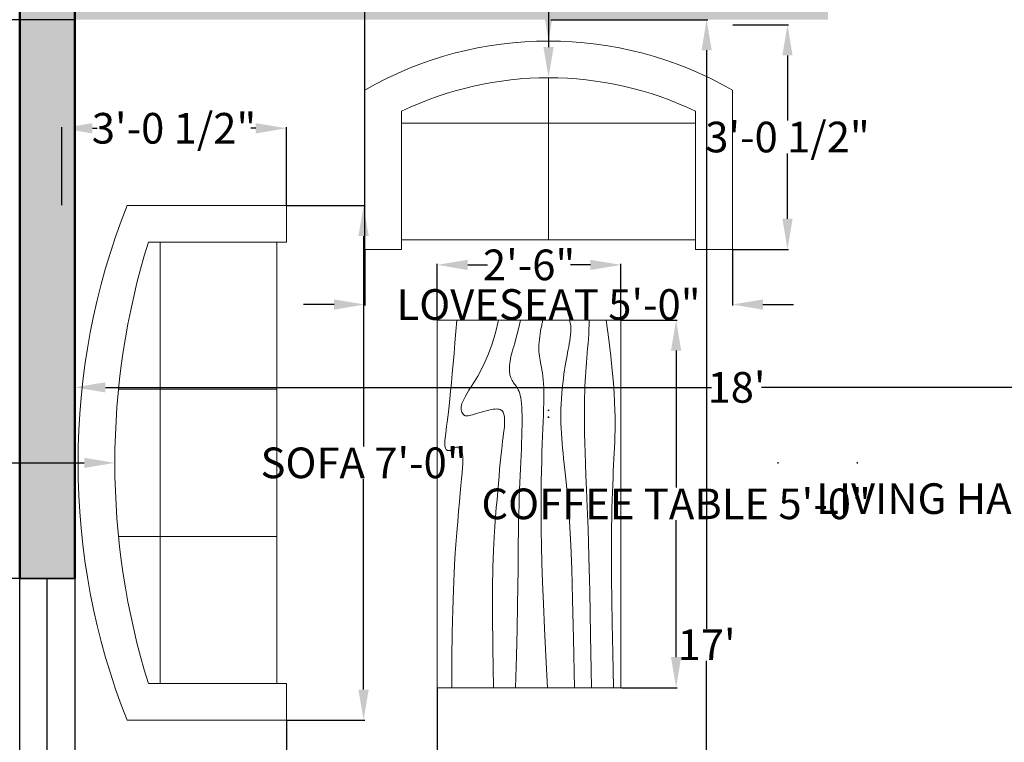
# Model space of a CAD drawing. Units: inches. Extents: x 3136 to 3620, y 13606 to 14152.
# Tile 3 of 6: x 3225 to 3386, y 13734 to 13852. Entities that reach past the tile are written whole.
import ezdxf

# ---------------------------------------------------------------- set-up
doc = ezdxf.new("R2010")
doc.units = ezdxf.units.IN
for name, color, linetype, lineweight in [('A-ANNO-DIMS', 2, 'Continuous', 18), ('A-AREA-IDEN', 7, 'Continuous', 25), ('A-FURN', 8, 'Continuous', 18), ('A-GLAZ', 4, 'Continuous', 25), ('A-WALL', 7, 'Continuous', 50), ('A-WALL-PATT', 174, 'Continuous', 13)]:
    doc.layers.add(name, color=color, linetype=linetype, lineweight=lineweight)
doc.styles.get("Standard").update_dxf_attribs({"font": 'arial.ttf', "height": 5})
doc.dimstyles.get("Standard").update_dxf_attribs({"dimtxt": 5, "dimasz": 5, "dimexe": 0.18, "dimexo": 0.0625, "dimgap": 0.09, "dimtad": 0, "dimtih": 1, "dimtoh": 1, "dimdec": 0, "dimzin": 0, "dimdsep": 46, "dimlunit": 3, "dimtxsty": 'Standard', "dimcen": 0.09, "dimadec": 0, "dimazin": 0, "dimtfac": 1, "dimtdec": 0, "dimtofl": 0, "dimtmove": 0, "dimatfit": 3, "dimfxl": 1, "dimtolj": 1, "dimtzin": 0, "dimarcsym": 0})

# ---------------------------------------------------------------- blocks, each defined once
blk = doc.blocks.new('*D15')
at = {"layer": 'A-ANNO-DIMS', "color": 0, "lineweight": -2, "transparency": 16777216}
for p, q in [((3233.87, 13788.87), (3233.87, 13792.02)), ((3238.87, 13791.84), (3337.77, 13791.84)), ((3444.87, 13791.84), (3345.97, 13791.84)), ((3449.87, 13788.87), (3449.87, 13792.02))]:
    blk.add_line(p, q, dxfattribs=at)
at = {"layer": 'A-ANNO-DIMS', "color": 0, "transparency": 16777216}
for points in [[(3238.87, 13792.67), (3238.87, 13791.01), (3233.87, 13791.84)], [(3444.87, 13792.67), (3444.87, 13791.01), (3449.87, 13791.84)]]:
    blk.add_solid(points, dxfattribs=at)
at = {"layer": 'Defpoints', "color": 0, "transparency": 16777216}
for p in [(3449.87, 13791.84), (3233.87, 13788.8), (3449.87, 13788.8)]:
    blk.add_point(p, dxfattribs=at)
at = {"layer": 'A-ANNO-DIMS', "color": 0, "transparency": 16777216, "insert": (3341.87, 13791.84), "char_height": 5, "attachment_point": 5}
blk.add_mtext("\\A1;18'", dxfattribs=at)
blk = doc.blocks.new('*D16')
at = {"layer": 'A-ANNO-DIMS', "color": 0, "lineweight": -2, "transparency": 16777216}
for p, q in [((3311.54, 13851.84), (3337.17, 13851.84)), ((3336.99, 13846.84), (3336.99, 13752.44)), ((3336.99, 13652.84), (3336.99, 13747.24)), ((3311.54, 13647.84), (3337.17, 13647.84))]:
    blk.add_line(p, q, dxfattribs=at)
at = {"layer": 'A-ANNO-DIMS', "color": 0, "transparency": 16777216}
for points in [[(3336.16, 13846.84), (3337.82, 13846.84), (3336.99, 13851.84)], [(3336.16, 13652.84), (3337.82, 13652.84), (3336.99, 13647.84)]]:
    blk.add_solid(points, dxfattribs=at)
at = {"layer": 'Defpoints', "color": 0, "transparency": 16777216}
for p in [(3311.47, 13851.84), (3336.99, 13851.84), (3311.47, 13647.84)]:
    blk.add_point(p, dxfattribs=at)
at = {"layer": 'A-ANNO-DIMS', "color": 0, "transparency": 16777216, "insert": (3336.99, 13749.84), "char_height": 5, "attachment_point": 5}
blk.add_mtext("\\A1;17'", dxfattribs=at)
blk = doc.blocks.new('Table - Rectangular Woodgrain 60 x 30 in.')
for p, q in [((0, 0), (0, -30)), ((60, 0), (0, 0)), ((60, -30), (60, 0)), ((0, -30), (60, -30))]:
    blk.add_line(p, q)
for points in [[(0, -2.4), (4.8155, -2.418), (9.0302, -2.4688), (12.709, -2.5477), (15.9167, -2.65), (18.7181, -2.7711), (21.1781, -2.9063), (23.3616, -3.0508), (25.3333, -3.2), (27.1477, -3.3495), (28.8172, -3.4958), (30.3437, -3.636), (31.7291, -3.7667), (32.9756, -3.8849), (34.0849, -3.9875), (35.059, -4.0714), (35.9, -4.1334), (36.6114, -4.1711), (37.2041, -4.1854), (37.6906, -4.1779), (38.0833, -4.15), (38.3948, -4.1034), (38.6375, -4.0396), (38.8239, -3.9602), (38.9666, -3.8667), (39.0764, -3.7608), (39.1573, -3.6448), (39.2116, -3.521), (39.2416, -3.3917), (39.2498, -3.2593), (39.2385, -3.1261), (39.21, -2.9944), (39.1666, -2.8667), (39.111, -2.7447), (39.0468, -2.6281), (38.978, -2.5163), (38.9083, -2.4083), (38.8418, -2.3035), (38.7823, -2.201), (38.7337, -2.1001), (38.7, -2), (38.6844, -1.9003), (38.6875, -1.8021), (38.7094, -1.707), (38.75, -1.6167), (38.8094, -1.5326), (38.8875, -1.4563), (38.9844, -1.3893), (39.1, -1.3333), (39.2351, -1.2896), (39.3937, -1.2583), (39.5804, -1.2396), (39.8, -1.2333), (40.057, -1.2396), (40.3562, -1.2583), (40.7023, -1.2896), (41.1, -1.3333), (41.5547, -1.3895), (42.0755, -1.4573), (42.6721, -1.5361), (43.3542, -1.625), (44.1316, -1.7233), (45.014, -1.8302), (46.0114, -1.9449), (47.1333, -2.0667), (48.3862, -2.1947), (49.7625, -2.3281), (51.2513, -2.4663), (52.8416, -2.6083), (54.5226, -2.7535), (56.2833, -2.9011), (58.1127, -3.0501), (60, -3.2)], [(0, -9.2), (6.5759, -9.0858), (11.9385, -9.0365), (16.2527, -9.0418), (19.6833, -9.0917), (22.3952, -9.1759), (24.5531, -9.2844), (26.322, -9.4069), (27.8666, -9.5333), (29.3241, -9.6553), (30.7203, -9.7719), (32.0532, -9.8837), (33.3208, -9.9917), (34.5213, -10.0965), (35.6526, -10.199), (36.7128, -10.2999), (37.7, -10.4), (38.6129, -10.4996), (39.4531, -10.5969), (40.223, -10.6895), (40.925, -10.775), (41.5613, -10.8512), (42.1344, -10.9156), (42.6465, -10.966), (43.1, -11), (43.4976, -11.0158), (43.8437, -11.0136), (44.143, -10.9942), (44.4, -10.9583), (44.6195, -10.9069), (44.8062, -10.8406), (44.9648, -10.7603), (45.1, -10.6667), (45.2155, -10.5598), (45.3114, -10.4365), (45.3871, -10.2929), (45.4416, -10.125), (45.4743, -9.929), (45.4844, -9.7011), (45.4709, -9.4371), (45.4333, -9.1333), (45.3716, -8.7883), (45.2896, -8.4104), (45.1919, -8.0107), (45.0833, -7.6), (44.9685, -7.1893), (44.8521, -6.7896), (44.7388, -6.4117), (44.6333, -6.0667), (44.54, -5.7628), (44.4614, -5.4979), (44.4001, -5.2675), (44.3583, -5.0667), (44.3384, -4.8909), (44.3427, -4.7354), (44.3736, -4.5956), (44.4333, -4.4667), (44.5236, -4.3453), (44.6427, -4.2333), (44.7884, -4.1339), (44.9583, -4.05), (45.1501, -3.9849), (45.3614, -3.9417), (45.59, -3.9234), (45.8333, -3.9333), (46.0915, -3.9749), (46.3734, -4.0531), (46.6906, -4.1736), (47.0542, -4.3417), (47.4756, -4.5629), (47.9661, -4.8427), (48.5372, -5.1866), (49.2, -5.6), (49.9676, -6.0844), (50.8594, -6.625), (51.8965, -7.2031), (53.1, -7.8), (54.491, -8.3969), (56.0906, -8.975), (57.9199, -9.5156), (60, -10)], [(0, -12.8), (5.1847, -12.9322), (9.6213, -13.0323), (13.3963, -13.1059), (16.5958, -13.1583), (19.3063, -13.1952), (21.614, -13.2219), (23.6054, -13.2439), (25.3666, -13.2667), (26.9728, -13.2947), (28.4531, -13.3281), (29.8256, -13.3663), (31.1083, -13.4083), (32.3191, -13.4535), (33.476, -13.501), (34.597, -13.5501), (35.7, -13.6), (36.7984, -13.6497), (37.8875, -13.6979), (38.9578, -13.743), (40, -13.7833), (41.0047, -13.8174), (41.9625, -13.8438), (42.864, -13.8607), (43.7, -13.8667), (44.4631, -13.8604), (45.1552, -13.8417), (45.7801, -13.8104), (46.3416, -13.7667), (46.8439, -13.7104), (47.2906, -13.6417), (47.6858, -13.5604), (48.0333, -13.4667), (48.3375, -13.3608), (48.6042, -13.2448), (48.8396, -13.121), (49.05, -12.9917), (49.2417, -12.8593), (49.4208, -12.7261), (49.5937, -12.5944), (49.7667, -12.4667), (49.9452, -12.3451), (50.1323, -12.2313), (50.3303, -12.1268), (50.5416, -12.0333), (50.7686, -11.9524), (51.0135, -11.8854), (51.2788, -11.8341), (51.5666, -11.8), (51.8785, -11.7843), (52.2116, -11.7865), (52.562, -11.8059), (52.926, -11.8417), (53.2998, -11.8931), (53.6795, -11.9594), (54.0614, -12.0397), (54.4416, -12.1333), (54.8223, -12.2401), (55.2293, -12.3625), (55.6942, -12.5037), (56.2489, -12.6667), (56.9251, -12.8547), (57.7545, -13.0708), (58.7689, -13.3182), (60, -13.6)], [(0, -18), (5.124, -17.7273), (9.6609, -17.5057), (13.6705, -17.3303), (17.2125, -17.1958), (20.3467, -17.0973), (23.1328, -17.0297), (25.6307, -16.9878), (27.9, -16.9667), (29.9928, -16.9617), (31.9302, -16.9703), (33.7254, -16.9907), (35.3917, -17.0208), (36.9423, -17.0588), (38.3906, -17.1026), (39.7499, -17.1503), (41.0333, -17.2), (42.2519, -17.2496), (43.4073, -17.2969), (44.4986, -17.3395), (45.525, -17.375), (46.4858, -17.4012), (47.3802, -17.4156), (48.2074, -17.416), (48.9667, -17.4), (49.6583, -17.3662), (50.2872, -17.3167), (50.8595, -17.2547), (51.3812, -17.1833), (51.8584, -17.1057), (52.2971, -17.025), (52.7034, -16.9443), (53.0833, -16.8667), (53.443, -16.7951), (53.789, -16.7313), (54.128, -16.6768), (54.4666, -16.6334), (54.8115, -16.6024), (55.1693, -16.5854), (55.5465, -16.5841), (55.95, -16.6), (56.3828, -16.6337), (56.8346, -16.6823), (57.2915, -16.7418), (57.7396, -16.8084), (58.165, -16.878), (58.5539, -16.9469), (58.8924, -17.0111), (59.1666, -17.0667), (59.3679, -17.1107), (59.5078, -17.1438), (59.6032, -17.1675), (59.6708, -17.1833), (59.7275, -17.193), (59.7901, -17.1979), (59.8753, -17.1998), (60, -17.2)], [(0, -22.4), (8.0098, -22.2501), (14.4094, -22.1011), (19.4168, -21.9535), (23.25, -21.8083), (26.1269, -21.6663), (28.2656, -21.5281), (29.884, -21.3947), (31.2, -21.2667), (32.3967, -21.1448), (33.5172, -21.0292), (34.5697, -20.9198), (35.5625, -20.8167), (36.5037, -20.7198), (37.4015, -20.6292), (38.2642, -20.5448), (39.1, -20.4667), (39.9164, -20.3951), (40.7187, -20.3313), (41.5117, -20.2768), (42.3, -20.2333), (43.0883, -20.2024), (43.8812, -20.1854), (44.6836, -20.1841), (45.5, -20.2), (46.3328, -20.234), (47.1747, -20.2844), (48.0163, -20.3488), (48.8479, -20.425), (49.66, -20.5106), (50.4429, -20.6031), (51.1872, -20.7004), (51.8833, -20.8), (52.5246, -20.8999), (53.1166, -20.9995), (53.6681, -21.0983), (54.1875, -21.1958), (54.6834, -21.2919), (55.1646, -21.3859), (55.6394, -21.4777), (56.1167, -21.5667), (56.6028, -21.6515), (57.0961, -21.7266), (57.5929, -21.7852), (58.0896, -21.8208), (58.5823, -21.8268), (59.0674, -21.7964), (59.5412, -21.723), (60, -21.6)], [(0, -25.2), (8.6355, -25.0504), (15.7026, -24.9031), (21.4049, -24.7606), (25.9458, -24.625), (29.529, -24.4988), (32.3578, -24.3844), (34.6359, -24.284), (36.5667, -24.2), (38.3213, -24.1341), (39.9417, -24.0854), (41.437, -24.0523), (42.8167, -24.0333), (44.0901, -24.0268), (45.2667, -24.0313), (46.3557, -24.0451), (47.3667, -24.0667), (48.309, -24.0947), (49.1928, -24.1287), (50.0284, -24.168), (50.826, -24.2125), (51.5959, -24.2617), (52.3483, -24.3151), (53.0935, -24.3725), (53.8417, -24.4334), (54.6009, -24.497), (55.3699, -24.561), (56.1454, -24.6226), (56.9239, -24.6792), (57.7021, -24.7279), (58.4764, -24.7662), (59.2435, -24.7911), (60, -24.8)], [(0, -28.8), (5.6867, -28.6681), (10.45, -28.5698), (14.407, -28.5012), (17.675, -28.4584), (20.3711, -28.4374), (22.6125, -28.4344), (24.5164, -28.4455), (26.2, -28.4667), (27.762, -28.4947), (29.2276, -28.5281), (30.6033, -28.5663), (31.8958, -28.6084), (33.1118, -28.6535), (34.2578, -28.7011), (35.3405, -28.7501), (36.3666, -28.8), (37.3443, -28.8497), (38.288, -28.8974), (39.2137, -28.9412), (40.1375, -28.9792), (41.0753, -29.0093), (42.0432, -29.0297), (43.0572, -29.0384), (44.1333, -29.0333), (45.2936, -29.0114), (46.5843, -28.9641), (48.0579, -28.8816), (49.7666, -28.7542), (51.7629, -28.5721), (54.0989, -28.3255), (56.8272, -28.0048), (60, -27.6)]]:
    blk.add_lwpolyline(points)
blk = doc.blocks.new('Sofa - Roundback 7 ft.')
for p, q in [((-12.00002, -32.4421), (-12.00003, -6.5971)), ((11.99997, -32.4421), (11.99998, -6.5971)), ((-36.000027, -34), (-36.000027, -11.4696)), ((35.99998, -34), (35.99998, -11.4696)), ((-35.999844, -13.3819), (35.9998, -13.3819)), ((-36.000027, -32.4421), (35.99998, -32.4421))]:
    blk.add_line(p, q)
for points in [[(-36.000027, -34), (-42.000027, -34), (-42.000027, -8)], [(41.99998, -8), (41.99998, -34), (35.99998, -34)]]:
    blk.add_lwpolyline(points)
for centre, radius, start, end in [((0, -114.25), 114.25, 68.43141, 111.5686), ((-0.00001, -127.1968), 121.1968, 72.72033, 107.2797)]:
    blk.add_arc(centre, radius, start, end)
blk = doc.blocks.new('Sofa - Roundback Loveseat 5 ft.')
for p, q in [((0, -32.44198), (0, -5.99998)), ((-24, -33.99998), (-24, -11.46958)), ((24.00004, -33.99998), (24.00004, -11.46958)), ((-23.9998, -13.38178), (23.99986, -13.38178)), ((-24, -32.44198), (24.00004, -32.44198))]:
    blk.add_line(p, q)
for points in [[(-24, -33.99998), (-30, -33.99998), (-30, -7.99998)], [(30.00004, -7.99998), (30.00004, -33.99998), (24.00004, -33.99998)]]:
    blk.add_lwpolyline(points)
for centre, radius, start, end in [((0, -60.24998), 60.24998, 60.13715, 119.8628), ((0, -61.38438), 55.38444, 64.32083, 115.6792)]:
    blk.add_arc(centre, radius, start, end)
blk = doc.blocks.new('*D28')
at = {"layer": 'A-ANNO-DIMS', "color": 0, "lineweight": -2, "transparency": 16777216}
for p, q in [((3224.81, 14118.84), (3200.37, 14118.84)), ((3200.55, 14113.84), (3200.55, 13881.48)), ((3200.55, 13643.84), (3200.55, 13876.2)), ((3224.81, 13638.84), (3200.37, 13638.84))]:
    blk.add_line(p, q, dxfattribs=at)
at = {"layer": 'A-ANNO-DIMS', "color": 0, "transparency": 16777216}
for points in [[(3199.71, 14113.84), (3201.38, 14113.84), (3200.55, 14118.84)], [(3199.71, 13643.84), (3201.38, 13643.84), (3200.55, 13638.84)]]:
    blk.add_solid(points, dxfattribs=at)
at = {"layer": 'Defpoints', "color": 0, "transparency": 16777216}
for p in [(3200.55, 14118.84), (3224.87, 14118.84), (3224.87, 13638.84)]:
    blk.add_point(p, dxfattribs=at)
at = {"layer": 'A-ANNO-DIMS', "color": 0, "transparency": 16777216, "insert": (3200.55, 13878.84), "char_height": 5, "attachment_point": 5}
blk.add_mtext("\\A1;40'", dxfattribs=at)
blk = doc.blocks.new('*D34')
at = {"layer": 'A-ANNO-DIMS', "color": 0, "lineweight": -2, "transparency": 16777216}
for p, q in [((3323.07, 13802.83), (3332.19, 13802.83)), ((3332.01, 13797.83), (3332.01, 13775.5)), ((3332.01, 13747.83), (3332.01, 13770.15)), ((3323.07, 13742.83), (3332.19, 13742.83))]:
    blk.add_line(p, q, dxfattribs=at)
at = {"layer": 'A-ANNO-DIMS', "color": 0, "transparency": 16777216}
for points in [[(3331.17, 13797.83), (3332.84, 13797.83), (3332.01, 13802.83)], [(3331.17, 13747.83), (3332.84, 13747.83), (3332.01, 13742.83)]]:
    blk.add_solid(points, dxfattribs=at)
at = {"layer": 'Defpoints', "color": 0, "transparency": 16777216}
for p in [(3323.01, 13802.83), (3332.01, 13802.83), (3323.01, 13742.83)]:
    blk.add_point(p, dxfattribs=at)
at = {"layer": 'A-ANNO-DIMS', "color": 0, "transparency": 16777216, "insert": (3332.01, 13772.83), "char_height": 5, "attachment_point": 5}
blk.add_mtext('\\A1;COFFEE TABLE 5\'-0"', dxfattribs=at)
blk = doc.blocks.new('*D35')
at = {"layer": 'A-ANNO-DIMS', "color": 0, "lineweight": -2, "transparency": 16777216}
for p, q in [((3293.01, 13802.89), (3293.01, 13812.01)), ((3298.01, 13811.83), (3301.23, 13811.83)), ((3318.01, 13811.83), (3314.79, 13811.83)), ((3323.01, 13802.89), (3323.01, 13812.01))]:
    blk.add_line(p, q, dxfattribs=at)
at = {"layer": 'A-ANNO-DIMS', "color": 0, "transparency": 16777216}
for points in [[(3298.01, 13812.66), (3298.01, 13810.99), (3293.01, 13811.83)], [(3318.01, 13812.66), (3318.01, 13810.99), (3323.01, 13811.83)]]:
    blk.add_solid(points, dxfattribs=at)
at = {"layer": 'Defpoints', "color": 0, "transparency": 16777216}
for p in [(3293.01, 13811.83), (3293.01, 13802.83), (3323.01, 13802.83)]:
    blk.add_point(p, dxfattribs=at)
at = {"layer": 'A-ANNO-DIMS', "color": 0, "transparency": 16777216, "insert": (3308.01, 13811.83), "char_height": 5, "attachment_point": 5}
blk.add_mtext('\\A1;2\'-6"', dxfattribs=at)
blk = doc.blocks.new('*D36')
at = {"layer": 'A-ANNO-DIMS', "color": 0, "lineweight": -2, "transparency": 16777216}
for p, q in [((3268.46, 13821.52), (3281.18, 13821.52)), ((3281, 13816.52), (3281, 13782.19)), ((3281, 13742.52), (3281, 13776.84)), ((3268.46, 13737.52), (3281.18, 13737.52))]:
    blk.add_line(p, q, dxfattribs=at)
at = {"layer": 'A-ANNO-DIMS', "color": 0, "transparency": 16777216}
for points in [[(3280.16, 13816.52), (3281.83, 13816.52), (3281, 13821.52)], [(3280.16, 13742.52), (3281.83, 13742.52), (3281, 13737.52)]]:
    blk.add_solid(points, dxfattribs=at)
at = {"layer": 'Defpoints', "color": 0, "transparency": 16777216}
for p in [(3268.4, 13821.52), (3281, 13821.52), (3268.4, 13737.52)]:
    blk.add_point(p, dxfattribs=at)
at = {"layer": 'A-ANNO-DIMS', "color": 0, "transparency": 16777216, "insert": (3281, 13779.52), "char_height": 5, "attachment_point": 5}
blk.add_mtext('\\A1;SOFA 7\'-0"', dxfattribs=at)
blk = doc.blocks.new('*D37')
at = {"layer": 'A-ANNO-DIMS', "color": 0, "lineweight": -2, "transparency": 16777216}
for p, q in [((3231.73, 13821.58), (3231.73, 13834.3)), ((3236.73, 13834.12), (3237.51, 13834.12)), ((3263.4, 13834.12), (3262.62, 13834.12)), ((3268.4, 13821.58), (3268.4, 13834.3))]:
    blk.add_line(p, q, dxfattribs=at)
at = {"layer": 'A-ANNO-DIMS', "color": 0, "transparency": 16777216}
for points in [[(3236.73, 13834.95), (3236.73, 13833.28), (3231.73, 13834.12)], [(3263.4, 13834.95), (3263.4, 13833.28), (3268.4, 13834.12)]]:
    blk.add_solid(points, dxfattribs=at)
at = {"layer": 'Defpoints', "color": 0, "transparency": 16777216}
for p in [(3231.73, 13834.12), (3231.73, 13821.52), (3268.4, 13821.52)]:
    blk.add_point(p, dxfattribs=at)
at = {"layer": 'A-ANNO-DIMS', "color": 0, "transparency": 16777216, "insert": (3250.06, 13834.12), "char_height": 5, "attachment_point": 5}
blk.add_mtext('\\A1;3\'-0 1/2"', dxfattribs=at)
blk = doc.blocks.new('*D38')
at = {"layer": 'A-ANNO-DIMS', "color": 0, "lineweight": -2, "transparency": 16777216}
for p, q in [((3281.19, 13814.29), (3281.19, 13805.18)), ((3341.19, 13814.29), (3341.19, 13805.18)), ((3276.19, 13805.36), (3271.19, 13805.36)), ((3346.19, 13805.36), (3351.19, 13805.36))]:
    blk.add_line(p, q, dxfattribs=at)
at = {"layer": 'A-ANNO-DIMS', "color": 0, "transparency": 16777216}
for points in [[(3276.19, 13806.19), (3276.19, 13804.52), (3281.19, 13805.36)], [(3346.19, 13806.19), (3346.19, 13804.52), (3341.19, 13805.36)]]:
    blk.add_solid(points, dxfattribs=at)
at = {"layer": 'Defpoints', "color": 0, "transparency": 16777216}
for p in [(3281.19, 13814.36), (3341.19, 13814.36), (3341.19, 13805.36)]:
    blk.add_point(p, dxfattribs=at)
at = {"layer": 'A-ANNO-DIMS', "color": 0, "transparency": 16777216, "insert": (3311.19, 13805.36), "char_height": 5, "attachment_point": 5}
blk.add_mtext('\\A1;LOVESEAT 5\'-0"', dxfattribs=at)
blk = doc.blocks.new('*D39')
at = {"layer": 'A-ANNO-DIMS', "color": 0, "lineweight": -2, "transparency": 16777216}
for p, q in [((3341.25, 13851.02), (3350.37, 13851.02)), ((3350.19, 13846.02), (3350.19, 13835.37)), ((3350.19, 13819.36), (3350.19, 13830.01)), ((3341.25, 13814.36), (3350.37, 13814.36))]:
    blk.add_line(p, q, dxfattribs=at)
at = {"layer": 'A-ANNO-DIMS', "color": 0, "transparency": 16777216}
for points in [[(3349.36, 13846.02), (3351.02, 13846.02), (3350.19, 13851.02)], [(3349.36, 13819.36), (3351.02, 13819.36), (3350.19, 13814.36)]]:
    blk.add_solid(points, dxfattribs=at)
at = {"layer": 'Defpoints', "color": 0, "transparency": 16777216}
for p in [(3341.19, 13851.02), (3350.19, 13851.02), (3341.19, 13814.36)]:
    blk.add_point(p, dxfattribs=at)
at = {"layer": 'A-ANNO-DIMS', "color": 0, "transparency": 16777216, "insert": (3350.19, 13832.69), "char_height": 5, "attachment_point": 5}
blk.add_mtext('\\A1;3\'-0 1/2"', dxfattribs=at)
blk = doc.blocks.new('*D63')
at = {"layer": 'A-ANNO-DIMS', "color": 0, "lineweight": -2, "transparency": 16777216}
for p, q in [((3233.81, 13851.84), (3207.89, 13851.84)), ((3208.07, 13846.84), (3208.07, 13808.82)), ((3208.07, 13765.63), (3208.07, 13803.64)), ((3233.81, 13760.63), (3207.89, 13760.63))]:
    blk.add_line(p, q, dxfattribs=at)
at = {"layer": 'A-ANNO-DIMS', "color": 0, "transparency": 16777216}
for points in [[(3207.24, 13846.84), (3208.9, 13846.84), (3208.07, 13851.84)], [(3207.24, 13765.63), (3208.9, 13765.63), (3208.07, 13760.63)]]:
    blk.add_solid(points, dxfattribs=at)
at = {"layer": 'Defpoints', "color": 0, "transparency": 16777216}
for p in [(3208.07, 13851.84), (3233.87, 13851.84), (3233.87, 13760.63)]:
    blk.add_point(p, dxfattribs=at)
at = {"layer": 'A-ANNO-DIMS', "color": 0, "transparency": 16777216, "insert": (3208.07, 13806.23), "char_height": 5, "attachment_point": 5}
blk.add_mtext('\\A1;7\'-7"', dxfattribs=at)
blk = doc.blocks.new('*D76')
at = {"layer": 'A-ANNO-DIMS', "color": 0, "lineweight": -2, "transparency": 16777216}
for p, q in [((3293.01, 13742.77), (3293.01, 13612.86)), ((3268.4, 13737.45), (3268.4, 13612.86)), ((3273.4, 13613.04), (3288.01, 13613.04)), ((3293.01, 13613.04), (3298.01, 13613.04))]:
    blk.add_line(p, q, dxfattribs=at)
at = {"layer": 'A-ANNO-DIMS', "color": 0, "transparency": 16777216}
for points in [[(3273.4, 13613.87), (3273.4, 13612.21), (3268.4, 13613.04)], [(3288.01, 13613.87), (3288.01, 13612.21), (3293.01, 13613.04)]]:
    blk.add_solid(points, dxfattribs=at)
at = {"layer": 'Defpoints', "color": 0, "transparency": 16777216}
for p in [(3293.01, 13742.83), (3268.4, 13737.52), (3293.01, 13613.04)]:
    blk.add_point(p, dxfattribs=at)
at = {"layer": 'A-ANNO-DIMS', "color": 0, "transparency": 16777216, "insert": (3310.61, 13613.04), "char_height": 5, "attachment_point": 5}
blk.add_mtext('\\A1;2\'-0 1/2"', dxfattribs=at)
blk = doc.blocks.new('*D77')
at = {"layer": 'A-ANNO-DIMS', "color": 0, "lineweight": -2, "transparency": 16777216}
for p, q in [((3233.87, 13851.9), (3233.87, 14144.82)), ((3238.87, 14144.64), (3243.03, 14144.64)), ((3276.19, 14144.64), (3272.03, 14144.64)), ((3281.19, 13814.42), (3281.19, 14144.82))]:
    blk.add_line(p, q, dxfattribs=at)
at = {"layer": 'A-ANNO-DIMS', "color": 0, "transparency": 16777216}
for points in [[(3238.87, 14145.47), (3238.87, 14143.81), (3233.87, 14144.64)], [(3276.19, 14145.47), (3276.19, 14143.81), (3281.19, 14144.64)]]:
    blk.add_solid(points, dxfattribs=at)
at = {"layer": 'Defpoints', "color": 0, "transparency": 16777216}
for p in [(3233.87, 14144.64), (3233.87, 13851.84), (3281.19, 13814.36)]:
    blk.add_point(p, dxfattribs=at)
at = {"layer": 'A-ANNO-DIMS', "color": 0, "transparency": 16777216, "insert": (3257.53, 14144.64), "char_height": 5, "attachment_point": 5}
blk.add_mtext('\\A1;3\'-11 1/2"', dxfattribs=at)
blk = doc.blocks.new('*D78')
at = {"layer": 'A-ANNO-DIMS', "color": 0, "lineweight": -2, "transparency": 16777216}
for p, q in [((3167.68, 13779.52), (3235.4, 13779.52)), ((3361.5, 13779.52), (3361.68, 13779.52)), ((3361.59, 13779.43), (3361.59, 13779.61))]:
    blk.add_line(p, q, dxfattribs=at)
at = {"layer": 'A-ANNO-DIMS', "color": 0, "transparency": 16777216}
blk.add_solid([(3235.4, 13780.35), (3235.4, 13778.68), (3240.4, 13779.52)], dxfattribs=at)
at = {"layer": 'Defpoints', "color": 0, "transparency": 16777216}
for p in [(3240.4, 13779.52), (3361.59, 13779.52)]:
    blk.add_point(p, dxfattribs=at)
at = {"layer": 'A-ANNO-DIMS', "color": 0, "transparency": 16777216, "insert": (3156.61, 13779.52), "char_height": 5, "attachment_point": 5}
blk.add_mtext('\\A1;R10\'-1"', dxfattribs=at)
blk = doc.blocks.new('*D79')
at = {"layer": 'A-ANNO-DIMS', "color": 0, "lineweight": -2, "transparency": 16777216}
for p, q in [((3165.85, 13779.52), (3229.4, 13779.52)), ((3348.56, 13779.52), (3348.74, 13779.52)), ((3348.65, 13779.43), (3348.65, 13779.61))]:
    blk.add_line(p, q, dxfattribs=at)
at = {"layer": 'A-ANNO-DIMS', "color": 0, "transparency": 16777216}
blk.add_solid([(3229.4, 13780.35), (3229.4, 13778.68), (3234.4, 13779.52)], dxfattribs=at)
at = {"layer": 'Defpoints', "color": 0, "transparency": 16777216}
for p in [(3234.4, 13779.52), (3348.65, 13779.52)]:
    blk.add_point(p, dxfattribs=at)
at = {"layer": 'A-ANNO-DIMS', "color": 0, "transparency": 16777216, "insert": (3150.89, 13779.52), "char_height": 5, "attachment_point": 5}
blk.add_mtext('\\A1;R9\'-6 1/2"', dxfattribs=at)
blk = doc.blocks.new('*D80')
at = {"layer": 'A-ANNO-DIMS', "color": 0, "lineweight": -2, "transparency": 16777216}
for p, q in [((3306.19, 13884.51), (3311.19, 13884.51)), ((3311.19, 13884.51), (3311.19, 13853.36)), ((3311.1, 13788.11), (3311.28, 13788.11)), ((3311.19, 13788.02), (3311.19, 13788.2))]:
    blk.add_line(p, q, dxfattribs=at)
at = {"layer": 'A-ANNO-DIMS', "color": 0, "transparency": 16777216}
blk.add_solid([(3312.02, 13853.36), (3310.36, 13853.36), (3311.19, 13848.36)], dxfattribs=at)
at = {"layer": 'Defpoints', "color": 0, "transparency": 16777216}
for p in [(3311.19, 13848.36), (3311.19, 13788.11)]:
    blk.add_point(p, dxfattribs=at)
at = {"layer": 'A-ANNO-DIMS', "color": 0, "transparency": 16777216, "insert": (3297.06, 13884.51), "char_height": 5, "attachment_point": 5}
blk.add_mtext('\\A1;R5\'-0"', dxfattribs=at)
blk = doc.blocks.new('*D81')
at = {"layer": 'A-ANNO-DIMS', "color": 0, "lineweight": -2, "transparency": 16777216}
for p, q in [((3306.19, 13875.59), (3311.19, 13875.59)), ((3311.19, 13875.59), (3311.19, 13847.36)), ((3311.19, 13786.88), (3311.19, 13787.06)), ((3311.1, 13786.97), (3311.28, 13786.97))]:
    blk.add_line(p, q, dxfattribs=at)
at = {"layer": 'A-ANNO-DIMS', "color": 0, "transparency": 16777216}
blk.add_solid([(3312.02, 13847.36), (3310.36, 13847.36), (3311.19, 13842.36)], dxfattribs=at)
at = {"layer": 'Defpoints', "color": 0, "transparency": 16777216}
for p in [(3311.19, 13842.36), (3311.19, 13786.97)]:
    blk.add_point(p, dxfattribs=at)
at = {"layer": 'A-ANNO-DIMS', "color": 0, "transparency": 16777216, "insert": (3291.24, 13875.59), "char_height": 5, "attachment_point": 5}
blk.add_mtext('\\A1;R4\'-7 1/2"', dxfattribs=at)

msp = doc.modelspace()

# ---------------------------------------------------------------- hatches: boundary and pattern name
at = {"layer": 'A-WALL-PATT'}
h = msp.add_hatch(color=256, dxfattribs=at)
h.dxf.hatch_style = 1
h.paths.add_polyline_path([(3584.87, 13767.84), (3575.87, 13767.84), (3575.87, 13714.7), (3584.87, 13714.7)])
h.paths.add_polyline_path([(3584.87, 13666.7), (3575.87, 13666.7), (3575.87, 13647.84), (3398.03, 13647.84), (3398.03, 13638.84), (3584.87, 13638.84)])
h.paths.add_polyline_path([(3350.03, 13647.84), (3272.91, 13647.84, -0.03225), (3273.24, 13642.78), (3273.24, 13638.84), (3350.03, 13638.84)])
h.paths.add_polyline_path([(3233.87, 13724.63), (3224.87, 13724.63), (3224.87, 13638.84), (3233.87, 13638.84), (3233.87, 13642.78), (3233.87, 13682.15)])
h.paths.add_polyline_path([(3233.87, 13893.84), (3224.87, 13893.84), (3224.87, 13760.63), (3233.87, 13760.63)])
h.paths.add_polyline_path([(3356.82, 13857.84), (3233.87, 13857.84), (3233.87, 13851.84), (3356.82, 13851.84)])
h.paths.add_polyline_path([(3233.87, 14022.84), (3224.87, 14022.84), (3224.87, 13941.84), (3233.87, 13941.84)])
h.paths.add_polyline_path([(3311.51, 13983.84), (3233.87, 13983.84), (3233.87, 13977.84), (3311.51, 13977.84)])
h.paths.add_polyline_path([(3467.87, 14118.84), (3224.87, 14118.84), (3224.87, 14070.84), (3233.87, 14070.84), (3233.87, 14081.66), (3233.87, 14109.84), (3467.87, 14109.84)])
h.paths.add_polyline_path([(3575.87, 13935.84), (3435.35, 13935.84, -0.018734), (3435.43, 13933.78), (3435.43, 13929.84), (3575.87, 13929.84)])
h.paths.add_polyline_path([(3417.35, 13932.93), (3424.89, 13932.93), (3424.89, 13943.24), (3417.35, 13943.24)], flags=9)
h.paths.add_polyline_path([(3561.82, 13786.65), (3573.42, 13786.65), (3573.42, 13796.96), (3561.82, 13796.96)], flags=9)
h.paths.add_polyline_path([(3567.12, 13888.65), (3574.84, 13888.65), (3574.84, 13898.96), (3567.12, 13898.96)], flags=9)
h.paths.add_polyline_path([(3536.01, 13916.38), (3543.73, 13916.38), (3543.73, 13926.69), (3536.01, 13926.69)], flags=9)
h.paths.add_polyline_path([(3509.85, 13733.24), (3521.46, 13733.24), (3521.46, 13743.54), (3509.85, 13743.54)], flags=9)
h.paths.add_polyline_path([(3499.97, 13866.95), (3511.39, 13866.95), (3511.39, 13877.25), (3499.97, 13877.25)], flags=9)
h.paths.add_polyline_path([(3456.03, 13744.65), (3463.57, 13744.65), (3463.57, 13754.96), (3456.03, 13754.96)], flags=9)

# ---------------------------------------------------------------- linework, layer by layer
at = {"layer": 'A-GLAZ'}
for p, q in [((3233.87, 13760.63), (3224.87, 13760.63)), ((3229.37, 13724.63), (3229.37, 13760.63))]:
    msp.add_line(p, q, dxfattribs=at)
msp.add_lwpolyline([(3224.87, 13760.63), (3233.87, 13760.63), (3233.87, 13724.63), (3224.87, 13724.63)], close=True, dxfattribs=at)
at = {"layer": 'A-WALL'}
msp.add_line((3233.87, 13760.63), (3233.87, 13893.84), dxfattribs=at)
msp.add_lwpolyline([(3224.87, 13760.63), (3224.87, 13893.84)], dxfattribs=at)

# ---------------------------------------------------------------- block references
at = {"layer": 'A-FURN'}
msp.add_blockref('Sofa - Roundback Loveseat 5 ft.', (3311.19, 13848.36), dxfattribs=at)
at = {"layer": 'A-FURN', "rotation": 90}
for name, p in [('Sofa - Roundback 7 ft.', (3234.4, 13779.52)), ('Table - Rectangular Woodgrain 60 x 30 in.', (3293.01, 13742.83))]:
    msp.add_blockref(name, p, dxfattribs=at)

# ---------------------------------------------------------------- texts
at = {"layer": 'A-AREA-IDEN', "insert": (3354.86, 13776.18), "char_height": 5, "attachment_point": 1}
msp.add_mtext_dynamic_manual_height_columns('LIVING HALL', width=50.6869, gutter_width=25, heights=[0], dxfattribs=at)

# ---------------------------------------------------------------- dimensions: what is measured, and where the dimension line sits
at = {"layer": 'A-ANNO-DIMS'}
for base, p1, p2, override, picture, middle in [((3233.87, 14144.64), (3281.19, 13814.36), (3233.87, 13851.84), {"dimdec": 1, "dimlfac": 1, "dimrnd": 0, "dimzin": 1, "dimdsep": 46, "dimlunit": 4, "dimfrac": 2}, '*D77', (3257.53, 14144.64)), ((3449.87, 13791.84), (3233.87, 13788.8), (3449.87, 13788.8), {"dimclrd": 0, "dimclre": 0, "dimclrt": 0}, '*D15', (3341.87, 13791.84)), ((3293.01, 13613.04), (3268.4, 13737.52), (3293.01, 13742.83), {"dimdec": 1, "dimlfac": 1, "dimrnd": 0, "dimzin": 1, "dimdsep": 46, "dimlunit": 4, "dimfrac": 2}, '*D76', (3310.61, 13613.04))]:
    dim = msp.add_linear_dim(base=base, p1=p1, p2=p2, dimstyle='Standard', override=override, dxfattribs=at)
    dim.commit()
    dim.dimension.update_dxf_attribs({"geometry": picture, "text_midpoint": middle})
for base, p1, p2, angle, override, picture, middle in [((3200.55, 14118.84), (3224.87, 13638.84), (3224.87, 14118.84), 90, {"dimclrd": 0, "dimclre": 0, "dimclrt": 0}, '*D28', (3200.55, 13878.84)), ((3208.07, 13851.84), (3233.87, 13760.63), (3233.87, 13851.84), 90, {"dimdec": 1, "dimlfac": 1, "dimrnd": 0, "dimzin": 1, "dimdsep": 46, "dimlunit": 4, "dimfrac": 2}, '*D63', (3208.07, 13806.23)), ((3350.19, 13851.02), (3341.19, 13814.36), (3341.19, 13851.02), 90, {"dimdec": 1, "dimlfac": 1, "dimrnd": 0, "dimzin": 1, "dimdsep": 46, "dimlunit": 4, "dimfrac": 2}, '*D39', (3350.19, 13832.69)), ((3231.73, 13834.12), (3268.4, 13821.52), (3231.73, 13821.52), 180, {"dimdec": 1, "dimlfac": 1, "dimrnd": 0, "dimzin": 1, "dimdsep": 46, "dimlunit": 4, "dimfrac": 2}, '*D37', (3250.06, 13834.12)), ((3293.01, 13811.83), (3323.01, 13802.83), (3293.01, 13802.83), 180, {"dimdec": 1, "dimlfac": 1, "dimrnd": 0, "dimzin": 1, "dimdsep": 46, "dimlunit": 4, "dimfrac": 2}, '*D35', (3308.01, 13811.83))]:
    dim = msp.add_linear_dim(base=base, p1=p1, p2=p2, angle=angle, dimstyle='Standard', override=override, dxfattribs=at)
    dim.commit()
    dim.dimension.update_dxf_attribs({"geometry": picture, "text_midpoint": middle})
for center, mpoint, picture, middle in [((3311.18914, 13788.1075), (3311.189, 13848.35748), '*D80', (3297.06072, 13884.50746)), ((3311.19, 13786.97), (3311.19, 13842.36), '*D81', (3291.24, 13875.59)), ((3348.64777, 13779.517148), (3234.39777, 13779.517), '*D79', (3165.84777, 13779.5169112)), ((3361.59, 13779.52), (3240.4, 13779.52), '*D78', (3167.68, 13779.52))]:
    dim = msp.add_radius_dim(center=center, mpoint=mpoint, dimstyle='Standard', override={"dimdec": 1, "dimlfac": 1, "dimrnd": 0, "dimzin": 1, "dimdsep": 46, "dimlunit": 4, "dimfrac": 2}, dxfattribs=at)
    dim.commit()
    dim.dimension.update_dxf_attribs({"geometry": picture, "text_midpoint": middle, "dimtype": 164})
dim = msp.add_linear_dim(base=(3336.99, 13851.84), p1=(3311.47, 13647.84), p2=(3311.47, 13851.84), angle=90, dimstyle='Standard', override={"dimclrd": 0, "dimclre": 0, "dimclrt": 0}, dxfattribs=at)
dim.commit()
dim.dimension.update_dxf_attribs({"geometry": '*D16', "text_midpoint": (3336.99, 13749.84), "dimtype": 160})
for base, p1, p2, text, picture, middle in [((3281, 13821.52), (3268.4, 13737.52), (3268.4, 13821.52), 'SOFA <>', '*D36', (3281, 13779.52)), ((3332.01, 13802.83), (3323.01, 13742.83), (3323.01, 13802.83), 'COFFEE TABLE <>', '*D34', (3332.01, 13772.83))]:
    dim = msp.add_linear_dim(base=base, p1=p1, p2=p2, angle=90, text=text, dimstyle='Standard', override={"dimdec": 1, "dimlfac": 1, "dimrnd": 0, "dimzin": 1, "dimdsep": 46, "dimlunit": 4, "dimfrac": 2}, dxfattribs=at)
    dim.commit()
    dim.dimension.update_dxf_attribs({"geometry": picture, "text_midpoint": middle})
dim = msp.add_linear_dim(base=(3341.19, 13805.36), p1=(3281.19, 13814.36), p2=(3341.19, 13814.36), text='LOVESEAT <>', dimstyle='Standard', override={"dimdec": 1, "dimlfac": 1, "dimrnd": 0, "dimzin": 1, "dimdsep": 46, "dimlunit": 4, "dimfrac": 2}, dxfattribs=at)
dim.commit()
dim.dimension.update_dxf_attribs({"geometry": '*D38', "text_midpoint": (3311.19, 13805.36)})

doc.saveas('drawing.dxf')
